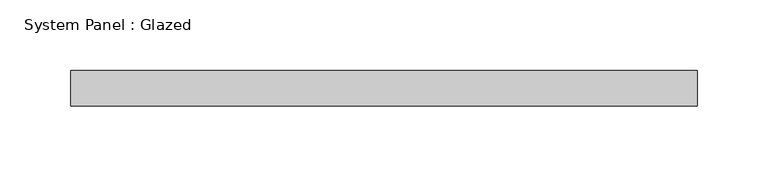
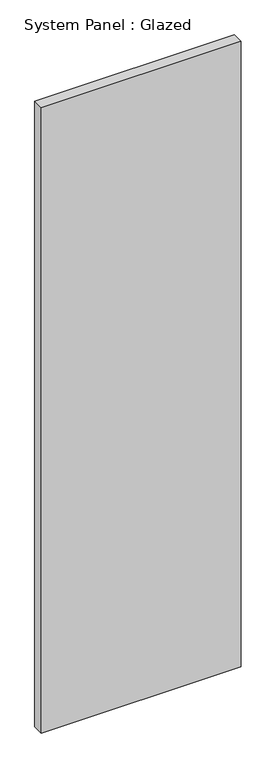
"""IFC4 building model written with IfcOpenShell, lengths in millimetres: plate geometry, System Panel : Glazed."""

from ifc_helpers import new_model, si_unit, origin, origin_with_axes, place, context, project, spatial, polyline, outline, extrude, source, transform, mapped, element, save


def system_panel_glazed_cd5540fc(model_context):
    return source(origin(), model_context, "Body", "SweptSolid", [
        extrude(outline(polyline([(222.25, 19.05), (-222.25, 19.05), (-222.25, 44.45), (222.25, 44.45), (222.25, 19.05)])), origin_with_axes(), (0.0, 0.0, 1.0), 1472.5620987),
    ])


if __name__ == "__main__":
    model = new_model("IFC4")
    model_context = context("Model", 3, world=origin())
    ifc_project = project(units=[si_unit("LENGTHUNIT", "METRE", prefix="MILLI")], contexts=[model_context])
    site = spatial("IfcSite", under=ifc_project)
    building = spatial("IfcBuilding", under=site)
    placement = place(None, origin())
    system_panel_glazed_shape = system_panel_glazed_cd5540fc(model_context)
    element("IfcPlate", 1, ObjectType="System Panel : Glazed", at=placement, inside=building, context=model_context, shape_type="MappedRepresentation", body=[
        mapped(system_panel_glazed_shape, transform((0.0, 0.0, 0.0), x_axis=(1.0, 0.0, 0.0), y_axis=(0.0, 1.0, 0.0), z_axis=(0.0, 0.0, 1.0))),
    ])
    save(model, "model.ifc")

# Revit data of these elements
# Type "System Panel : Glazed"
#   Construction Type Id = "GSP4R"
#   Analytic Construction = "1/8 in Pilkington single glazing"
#   Visual Light Transmittance = 0.9
#   Solar Heat Gain Coefficient = 0.86
#   Heat Transfer Coefficient (U) = 1.18115 BTU/(h·ft²·°F)
#   Define Thermal Properties by = 1
# Element 1 (IfcPlate, "System Panel : Glazed")
#   Materials on its faces: "Glass"
# Materials
#   "Glass": class "Glass", colour RGB 0 128 192, transparency 0.75, Description = "Soda Lime Glass", Cost = 0
